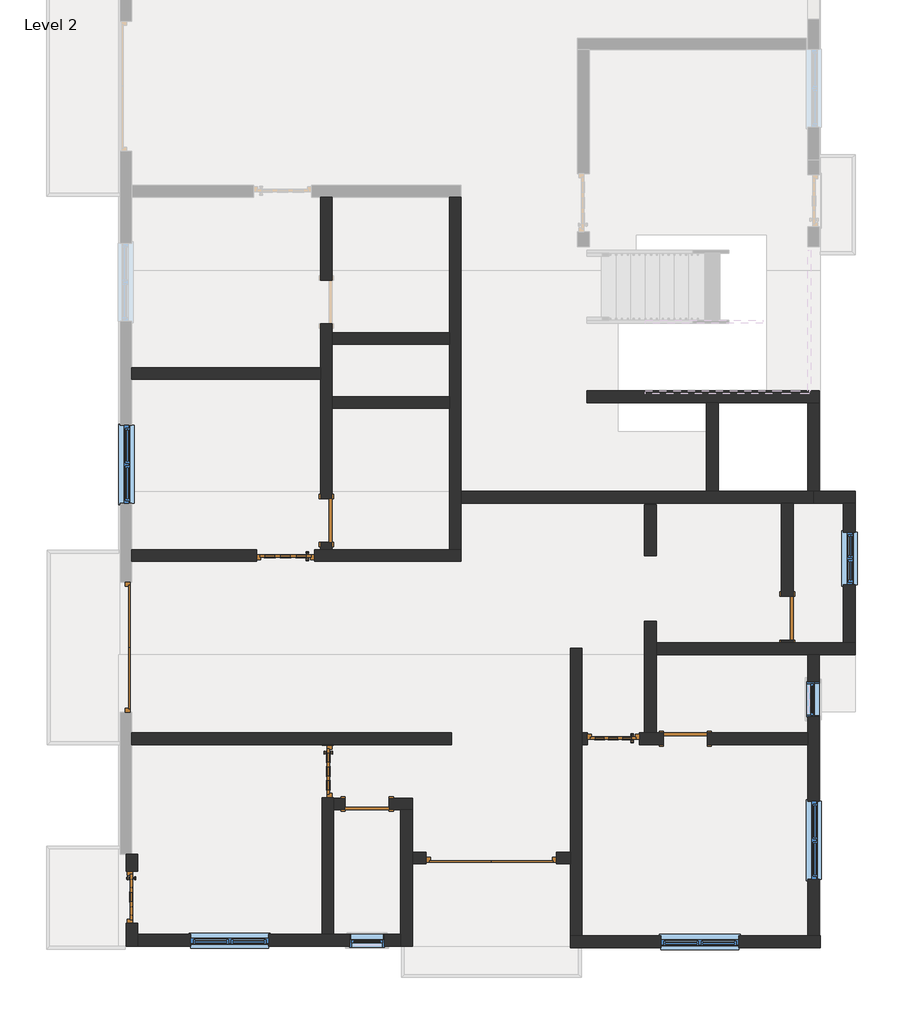
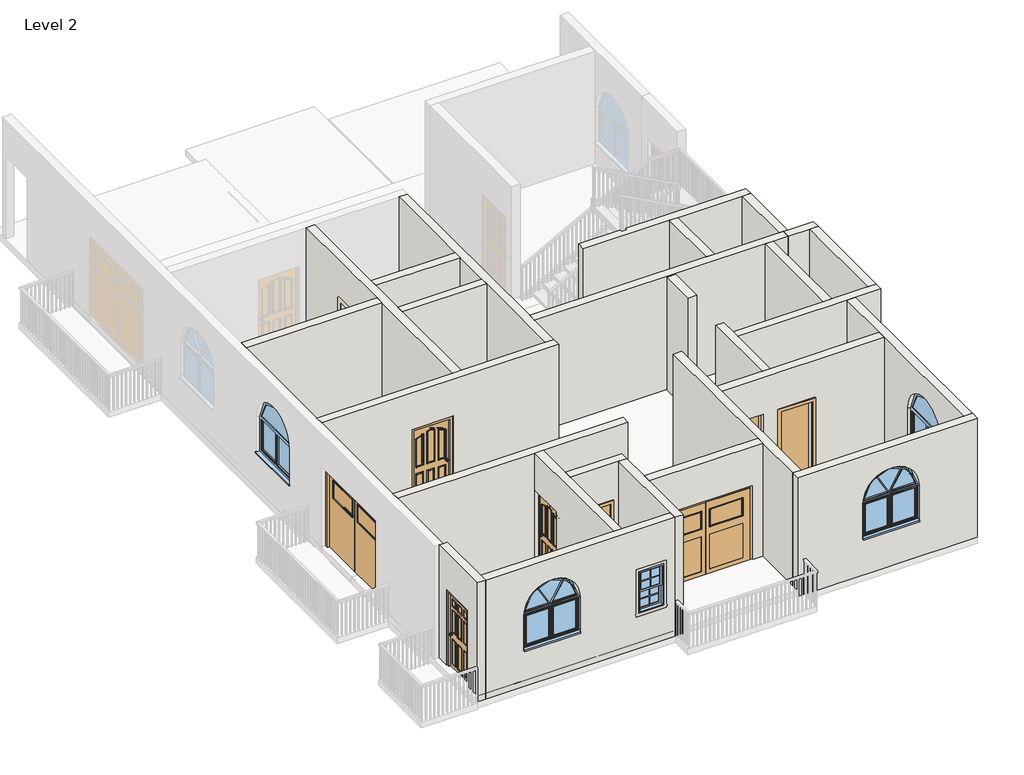
# One storey, part 1 of 7: 27 walls, 10 doors, 7 windows.
"""IFC4 building model written with IfcOpenShell, lengths in millimetres."""

from ifc_helpers import new_model, si_unit, frame, origin, place, context, project, spatial, polyline, circle_curve, outline, extrude, faceted_brep, transform, mapped, element, save
from ifc_brep_helpers import plane_surface, revolved_surface, advanced_brep
from components import doors_extsgl_5_910x2110mm_99758a98, doors_extsgl_6_1010x2110mm_b93c615f, doors_extsgl_6_1010x2110mm_efbaf1af, doors_extsgl_6_910x2110mm_72be2df1, doors_extsgl_6_910x2110mm_b26fcae4, doors_extsgl_6_910x2110mm_5dc58899, doors_extsgl_6_910x2110mm_16d7c084, doors_garage_timber_side_hung_glazing_2270x2050mm_ae99176d, doors_garage_timber_side_hung_glazing_2270x2200mm_badb7014, door_fadea3f2, door_53b1b562, window_679d2811, windows_arched_1360x910mm_c5754810, windows_dbl_w_glazing_bars_910x910mm_41eba874

model = new_model("IFC4")

# Units and contexts
model_context = context("Model", 3, world=origin())
ifc_project = project(units=[si_unit("LENGTHUNIT", "METRE", prefix="MILLI")], contexts=[model_context])

# Site, building, storey
site = spatial("IfcSite", under=ifc_project)
building = spatial("IfcBuilding", under=site)
storey = spatial("IfcBuildingStorey", under=building, Name="Level 2", Elevation=3048.0)

# Doors
placement = place(None, origin())
doors_extsgl_5_910x2110mm_shape = doors_extsgl_5_910x2110mm_99758a98(model_context)
element("IfcDoor", 1, ObjectType="Doors_ExtSgl_5 : 910x2110mm", at=placement, inside=storey, context=model_context, shape_type="MappedRepresentation", body=[
    mapped(doors_extsgl_5_910x2110mm_shape, transform((-6127.6013636, -9759.5108149, 3048.0), x_axis=(0.0, -1.0, 0.0), y_axis=(1.0, 0.0, 0.0), z_axis=(0.0, 0.0, 1.0))),
])
doors_extsgl_6_1010x2110mm_shape = doors_extsgl_6_1010x2110mm_b93c615f(model_context)
doors_extsgl_6_1010x2110mm_2_shape = doors_extsgl_6_1010x2110mm_efbaf1af(model_context)
element("IfcDoor", 2, ObjectType="Doors_ExtSgl_6 : 1010x2110mm", at=placement, inside=storey, context=model_context, shape_type="MappedRepresentation", body=[
    mapped(doors_extsgl_6_1010x2110mm_shape, transform((-3445.8775704, -3805.7037749, 3048.0), x_axis=(-1.0, 0.0, 0.0), y_axis=(0.0, -1.0, 0.0), z_axis=(0.0, 0.0, 1.0))),
    mapped(doors_extsgl_6_1010x2110mm_2_shape, transform((-3445.8775704, -3805.7037749, 3048.0), x_axis=(-1.0, 0.0, 0.0), y_axis=(0.0, -1.0, 0.0), z_axis=(0.0, 0.0, 1.0))),
])
doors_extsgl_6_910x2110mm_shape = doors_extsgl_6_910x2110mm_72be2df1(model_context)
doors_extsgl_6_910x2110mm_2_shape = doors_extsgl_6_910x2110mm_b26fcae4(model_context)
element("IfcDoor", 3, ObjectType="Doors_ExtSgl_6 : 910x2110mm", at=placement, inside=storey, context=model_context, shape_type="MappedRepresentation", body=[
    mapped(doors_extsgl_6_910x2110mm_shape, transform((2269.1224296, -6998.5466225, 3048.0), x_axis=(-1.0, 0.0, 0.0), y_axis=(0.0, -1.0, 0.0), z_axis=(0.0, 0.0, 1.0))),
    mapped(doors_extsgl_6_910x2110mm_2_shape, transform((2269.1224296, -6998.5466225, 3048.0), x_axis=(-1.0, 0.0, 0.0), y_axis=(0.0, -1.0, 0.0), z_axis=(0.0, 0.0, 1.0))),
])
doors_extsgl_6_910x2110mm_3_shape = doors_extsgl_6_910x2110mm_5dc58899(model_context)
doors_extsgl_6_910x2110mm_4_shape = doors_extsgl_6_910x2110mm_16d7c084(model_context)
element("IfcDoor", 4, ObjectType="Doors_ExtSgl_6 : 910x2110mm", at=placement, inside=storey, context=model_context, shape_type="MappedRepresentation", body=[
    mapped(doors_extsgl_6_910x2110mm_3_shape, transform((-2709.3109037, -7568.3747197, 3048.0), x_axis=(0.0, -1.0, 0.0), y_axis=(1.0, 0.0, 0.0), z_axis=(0.0, 0.0, 1.0))),
    mapped(doors_extsgl_6_910x2110mm_4_shape, transform((-2709.3109037, -7568.3747197, 3048.0), x_axis=(0.0, -1.0, 0.0), y_axis=(1.0, 0.0, 0.0), z_axis=(0.0, 0.0, 1.0))),
])
doors_garage_timber_side_hung_glazing_2270x2050mm_shape = doors_garage_timber_side_hung_glazing_2270x2050mm_ae99176d(model_context)
element("IfcDoor", 5, ObjectType="Doors_Garage_Timber_Side_Hung_Glazing : 2270x2050mm", at=placement, inside=storey, context=model_context, shape_type="MappedRepresentation", body=[
    mapped(doors_garage_timber_side_hung_glazing_2270x2050mm_shape, transform((141.8390963, -9078.0694836, 3048.0), x_axis=(-1.0, 0.0, 0.0), y_axis=(0.0, -1.0, 0.0), z_axis=(0.0, 0.0, 1.0))),
])
doors_garage_timber_side_hung_glazing_2270x2200mm_shape = doors_garage_timber_side_hung_glazing_2270x2200mm_badb7014(model_context)
element("IfcDoor", 6, ObjectType="Doors_Garage_Timber_Side_Hung_Glazing : 2270x2200mm", at=placement, inside=storey, context=model_context, shape_type="MappedRepresentation", body=[
    mapped(doors_garage_timber_side_hung_glazing_2270x2200mm_shape, transform((-6229.2013636, -5402.1251987, 3048.0), x_axis=(0.0, 1.0, 0.0), y_axis=(-1.0, 0.0, 0.0), z_axis=(0.0, 0.0, 1.0))),
])
door_shape = door_fadea3f2(model_context)
element("IfcDoor", 7, ObjectType="Single-Flush : 30\" x 80\"", at=placement, inside=storey, context=model_context, shape_type="MappedRepresentation", body=[
    mapped(door_shape, transform((-2023.5109037, -8138.2694836, 3048.0), x_axis=(-1.0, 0.0, 0.0), y_axis=(0.0, -1.0, 0.0), z_axis=(0.0, 0.0, 1.0))),
])
element("IfcDoor", 8, ObjectType="Single-Flush : 30\" x 80\"", at=placement, inside=storey, context=model_context, shape_type="MappedRepresentation", body=[
    mapped(door_shape, transform((5304.3890963, -4897.9037749, 3048.0), x_axis=(0.0, -1.0, 0.0), y_axis=(1.0, 0.0, 0.0), z_axis=(0.0, 0.0, 1.0))),
])
door_2_shape = door_53b1b562(model_context)
element("IfcDoor", 9, ObjectType="Single-Flush : 30\" x 80\"", at=placement, inside=storey, context=model_context, shape_type="MappedRepresentation", body=[
    mapped(door_2_shape, transform((-2734.7109037, -3196.1037749, 3048.0), x_axis=(0.0, 1.0, 0.0), y_axis=(-1.0, 0.0, 0.0), z_axis=(0.0, 0.0, 1.0))),
])
element("IfcDoor", 10, ObjectType="Single-Flush : 30\" x 80\"", at=placement, inside=storey, context=model_context, shape_type="MappedRepresentation", body=[
    mapped(door_2_shape, transform((3526.3890963, -6998.5466225, 3048.0), x_axis=(-1.0, 0.0, 0.0), y_axis=(0.0, -1.0, 0.0), z_axis=(0.0, 0.0, 1.0))),
])

# Walls
element("IfcWall", 11, ObjectType="Generic - 9\" w", at=placement, inside=storey, context=model_context, shape_type="Brep", body=[
    faceted_brep([(6485.4890963, -2688.1037749, 3048.0), (5863.1890963, -2688.1037749, 3048.0), (5761.5890963, -2688.1037749, 3048.0), (5761.5890963, -2688.1037749, 6096.0), (5863.1890963, -2688.1037749, 6096.0), (6485.4890963, -2688.1037749, 6096.0), (6485.4890963, -2891.3037749, 3048.0), (6485.4890963, -2891.3037749, 6096.0), (6282.2890963, -2891.3037749, 6096.0), (5761.5890963, -2891.3037749, 6096.0), (5761.5890963, -2891.3037749, 3048.0), (6282.2890963, -2891.3037749, 3048.0)], [[[0, 1, 2, 3, 4, 5]], [[6, 7, 8, 9, 10, 11]], [[2, 1, 0, 6, 11, 10]], [[3, 2, 10, 9]], [[5, 4, 3, 9, 8, 7]], [[0, 5, 7, 6]]]),
])
element("IfcWall", 12, ObjectType="Generic - 9\" w", at=placement, inside=storey, context=model_context, shape_type="Brep", body=[
    faceted_brep([(5761.5890963, -2688.1037749, 3048.0), (5659.9890963, -2688.1037749, 3048.0), (4097.8890963, -2688.1037749, 3048.0), (3894.6890963, -2688.1037749, 3048.0), (-385.2109037, -2688.1037749, 3048.0), (-385.2109037, -2688.1037749, 6096.0), (3894.6890963, -2688.1037749, 6096.0), (4097.8890963, -2688.1037749, 6096.0), (5659.9890963, -2688.1037749, 6096.0), (5761.5890963, -2688.1037749, 6096.0), (5761.5890963, -2891.3037749, 3048.0), (5761.5890963, -2891.3037749, 6096.0), (5405.9890963, -2891.3037749, 6096.0), (5202.7890963, -2891.3037749, 6096.0), (-385.2109037, -2891.3037749, 6096.0), (-385.2109037, -2891.3037749, 3048.0), (5202.7890963, -2891.3037749, 3048.0), (5405.9890963, -2891.3037749, 3048.0)], [[[0, 1, 2, 3, 4, 5, 6, 7, 8, 9]], [[10, 11, 12, 13, 14, 15, 16, 17]], [[4, 3, 2, 1, 0, 10, 17, 16, 15]], [[9, 8, 7, 6, 5, 14, 13, 12, 11]], [[0, 9, 11, 10]], [[5, 4, 15, 14]]]),
])
element("IfcWall", 13, ObjectType="Generic - 9\" w", at=placement, inside=storey, context=model_context, shape_type="SweptSolid", body=[
    extrude(outline(polyline([(3894.6890963, -2688.1037749), (3894.6890963, -1138.7037749), (4097.8890963, -1138.7037749), (4097.8890963, -2688.1037749), (3894.6890963, -2688.1037749)])), frame((0.0, 0.0, 3048.0), z_axis=(0.0, 0.0, 1.0), x_axis=(1.0, 0.0, 0.0)), (0.0, 0.0, 1.0), 3048.0),
])
element("IfcWall", 14, ObjectType="Generic - 9\" w", at=placement, inside=storey, context=model_context, shape_type="Brep", body=[
    faceted_brep([(5863.1890963, -935.5037749, 3048.0), (1812.4805171, -935.5037749, 3048.0), (1812.4805171, -935.5037749, 6096.0), (5863.1890963, -935.5037749, 6096.0), (5863.1890963, -1138.7037749, 3048.0), (5863.1890963, -1138.7037749, 6096.0), (5659.9890963, -1138.7037749, 6096.0), (4097.8890963, -1138.7037749, 6096.0), (3894.6890963, -1138.7037749, 6096.0), (1812.4805171, -1138.7037749, 6096.0), (1812.4805171, -1138.7037749, 3048.0), (3894.6890963, -1138.7037749, 3048.0), (4097.8890963, -1138.7037749, 3048.0), (5659.9890963, -1138.7037749, 3048.0)], [[[0, 1, 2, 3]], [[4, 5, 6, 7, 8, 9, 10, 11, 12, 13]], [[1, 0, 4, 13, 12, 11, 10]], [[2, 1, 10, 9]], [[3, 2, 9, 8, 7, 6, 5]], [[0, 3, 5, 4]]]),
])
element("IfcWall", 15, ObjectType="Generic - 9\" w", at=placement, inside=storey, context=model_context, shape_type="AdvancedBrep", body=[
    advanced_brep(
    [(1519.7890963, -10638.3037749, 3048.0), (5875.8890963, -10638.3037749, 3048.0), (5875.8890963, -10638.3037749, 6096.0), (1519.7890963, -10638.3037749, 6096.0), (4460.3890963, -10638.3037749, 3962.4), (3100.3890963, -10638.3037749, 3962.4), (3100.3890963, -10638.3037749, 4872.4), (4460.3890963, -10638.3037749, 4872.4), (1519.7890963, -10435.1037749, 3048.0), (1519.7890963, -10435.1037749, 6096.0), (1722.9890963, -10435.1037749, 6096.0), (5659.9890963, -10435.1037749, 6096.0), (5863.1890963, -10435.1037749, 6096.0), (5875.8890963, -10435.1037749, 6096.0), (5875.8890963, -10435.1037749, 3048.0), (5863.1890963, -10435.1037749, 3048.0), (5659.9890963, -10435.1037749, 3048.0), (1722.9890963, -10435.1037749, 3048.0), (4460.3890963, -10435.1037749, 3962.4), (4460.3890963, -10435.1037749, 4872.4), (3100.3890963, -10435.1037749, 4872.4), (3100.3890963, -10435.1037749, 3962.4)],
    [
        (0, 1),
        (1, 2),
        (2, 3),
        (3, 0),
        (4, 5),
        (5, 6),
        (6, 7, circle_curve(frame((3780.3890963, -10638.3037749, 4872.4), z_axis=(0.0, 1.0, 0.0), x_axis=(-1.0, 0.0, 0.0)), 680.0)),
        (7, 4),
        (8, 9),
        (9, 10),
        (10, 11),
        (11, 12),
        (12, 13),
        (13, 14),
        (14, 15),
        (15, 16),
        (16, 17),
        (17, 8),
        (18, 19),
        (19, 20, circle_curve(frame((3780.3890963, -10435.1037749, 4872.4), z_axis=(0.0, -1.0, 0.0), x_axis=(-1.0, 0.0, 0.0)), 680.0)),
        (20, 21),
        (21, 18),
        (0, 8),
        (14, 1),
        (13, 2),
        (9, 3),
        (18, 4),
        (7, 19),
        (6, 20),
        (5, 21),
    ],
    [
        plane_surface(frame((1722.9890963, -10638.3037749, 3048.0), z_axis=(0.0, -1.0, 0.0), x_axis=(1.0, 0.0, 0.0))),
        plane_surface(frame((1722.9890963, -10435.1037749, 3048.0), z_axis=(0.0, 1.0, 0.0), x_axis=(-1.0, 0.0, 0.0))),
        plane_surface(frame((1621.3890963, -10638.3037749, 3048.0), z_axis=(0.0, 0.0, -1.0), x_axis=(0.0, 1.0, 0.0))),
        plane_surface(frame((5875.8890963, -10638.3037749, 3048.0), z_axis=(1.0, 0.0, 0.0), x_axis=(0.0, 1.0, 0.0))),
        plane_surface(frame((5875.8890963, -10638.3037749, 6096.0), z_axis=(0.0, 0.0, 1.0), x_axis=(0.0, 1.0, 0.0))),
        plane_surface(frame((1519.7890963, -5418.6037749, 3048.0), z_axis=(-1.0, 0.0, 0.0), x_axis=(0.0, -1.0, 0.0))),
        plane_surface(frame((4460.3890963, -10435.1037749, 3962.4), z_axis=(-1.0, 0.0, 0.0), x_axis=(0.0, -1.0, 0.0))),
        revolved_surface(polyline([(3100.3890963, -10638.3037749, 4872.4), (3100.3890963, -10435.1037749, 4872.4)]), (3780.3890963, -10435.1037749, 4872.4), (0.0, -1.0, 0.0)),
        plane_surface(frame((3100.3890963, -10435.1037749, 4872.4), z_axis=(1.0, 0.0, 0.0), x_axis=(0.0, -1.0, 0.0))),
        plane_surface(frame((3100.3890963, -10435.1037749, 3962.4), z_axis=(0.0, 0.0, 1.0), x_axis=(0.0, -1.0, 0.0))),
    ],
    [
        (0, [[1, 2, 3, 4], [5, 6, 7, 8]]),
        (1, [[9, 10, 11, 12, 13, 14, 15, 16, 17, 18], [19, 20, 21, 22]]),
        (2, [[-1, 23, -18, -17, -16, -15, 24]]),
        (3, [[-2, -24, -14, 25]]),
        (4, [[-3, -25, -13, -12, -11, -10, 26]]),
        (5, [[-4, -26, -9, -23]]),
        (6, [[-19, 27, -8, 28]]),
        (7, [[-20, -28, -7, 29]]),
        (8, [[-21, -29, -6, 30]]),
        (9, [[-22, -30, -5, -27]]),
    ],
),
])
element("IfcWall", 16, ObjectType="Generic - 9\" w", at=placement, inside=storey, context=model_context, shape_type="AdvancedBrep", body=[
    advanced_brep(
    [(5863.1890963, -10435.1037749, 3048.0), (5863.1890963, -5532.9037749, 3048.0), (5863.1890963, -5532.9037749, 6096.0), (5863.1890963, -10435.1037749, 6096.0), (5863.1890963, -8087.6251987, 3962.4), (5863.1890963, -9447.6251987, 3962.4), (5863.1890963, -9447.6251987, 4872.4), (5863.1890963, -8087.6251987, 4872.4), (5863.1890963, -6618.7537749, 5029.2), (5863.1890963, -6009.1537749, 5029.2), (5863.1890963, -6009.1537749, 3962.4), (5863.1890963, -6618.7537749, 3962.4), (5659.9890963, -10435.1037749, 3048.0), (5659.9890963, -10435.1037749, 6096.0), (5659.9890963, -7100.1466225, 6096.0), (5659.9890963, -6896.9466225, 6096.0), (5659.9890963, -5532.9037749, 6096.0), (5659.9890963, -5532.9037749, 3048.0), (5659.9890963, -6896.9466225, 3048.0), (5659.9890963, -7100.1466225, 3048.0), (5659.9890963, -8087.6251987, 3962.4), (5659.9890963, -8087.6251987, 4872.4), (5659.9890963, -9447.6251987, 4872.4), (5659.9890963, -9447.6251987, 3962.4), (5659.9890963, -6618.7537749, 5029.2), (5659.9890963, -6618.7537749, 3962.4), (5659.9890963, -6009.1537749, 3962.4), (5659.9890963, -6009.1537749, 5029.2)],
    [
        (0, 1),
        (1, 2),
        (2, 3),
        (3, 0),
        (4, 5),
        (5, 6),
        (6, 7, circle_curve(frame((5863.1890963, -8767.6251987, 4872.4), z_axis=(-1.0, 0.0, 0.0), x_axis=(0.0, -1.0, 0.0)), 680.0)),
        (7, 4),
        (8, 9),
        (9, 10),
        (10, 11),
        (11, 8),
        (12, 13),
        (13, 14),
        (14, 15),
        (15, 16),
        (16, 17),
        (17, 18),
        (18, 19),
        (19, 12),
        (20, 21),
        (21, 22, circle_curve(frame((5659.9890963, -8767.6251987, 4872.4), z_axis=(1.0, 0.0, 0.0), x_axis=(0.0, -1.0, 0.0)), 680.0)),
        (22, 23),
        (23, 20),
        (24, 25),
        (25, 26),
        (26, 27),
        (27, 24),
        (0, 12),
        (17, 1),
        (2, 16),
        (13, 3),
        (20, 4),
        (7, 21),
        (6, 22),
        (5, 23),
        (24, 8),
        (11, 25),
        (10, 26),
        (9, 27),
    ],
    [
        plane_surface(frame((5863.1890963, -10435.1037749, 3048.0), z_axis=(1.0, 0.0, 0.0), x_axis=(0.0, 1.0, 0.0))),
        plane_surface(frame((5659.9890963, -10435.1037749, 3048.0), z_axis=(-1.0, 0.0, 0.0), x_axis=(0.0, -1.0, 0.0))),
        plane_surface(frame((5863.1890963, -10536.7037749, 3048.0), z_axis=(0.0, 0.0, -1.0), x_axis=(-1.0, 0.0, 0.0))),
        plane_surface(frame((5863.1890963, -5431.3037749, 6096.0), z_axis=(0.0, 0.0, 1.0), x_axis=(-1.0, 0.0, 0.0))),
        plane_surface(frame((1722.9890963, -10435.1037749, 3048.0), z_axis=(0.0, -1.0, 0.0), x_axis=(-1.0, 0.0, 0.0))),
        plane_surface(frame((3018.3890963, -5532.9037749, 3048.0), z_axis=(0.0, 1.0, 0.0), x_axis=(1.0, 0.0, 0.0))),
        plane_surface(frame((5659.9890963, -8087.6251987, 3962.4), z_axis=(0.0, -1.0, 0.0), x_axis=(1.0, 0.0, 0.0))),
        revolved_surface(polyline([(5863.1890963, -9447.6251987, 4872.4), (5659.9890963, -9447.6251987, 4872.4)]), (5659.9890963, -8767.6251987, 4872.4), (1.0, 0.0, 0.0)),
        plane_surface(frame((5659.9890963, -9447.6251987, 4872.4), z_axis=(0.0, 1.0, 0.0), x_axis=(1.0, 0.0, 0.0))),
        plane_surface(frame((5659.9890963, -9447.6251987, 3962.4), z_axis=(0.0, 0.0, 1.0), x_axis=(1.0, 0.0, 0.0))),
        plane_surface(frame((5659.9890963, -6618.7537749, 5029.2), z_axis=(0.0, 1.0, 0.0), x_axis=(1.0, 0.0, 0.0))),
        plane_surface(frame((5659.9890963, -6618.7537749, 3962.4), z_axis=(0.0, 0.0, 1.0), x_axis=(1.0, 0.0, 0.0))),
        plane_surface(frame((5659.9890963, -6009.1537749, 3962.4), z_axis=(0.0, -1.0, 0.0), x_axis=(1.0, 0.0, 0.0))),
        plane_surface(frame((5659.9890963, -6009.1537749, 5029.2), z_axis=(0.0, 0.0, -1.0), x_axis=(1.0, 0.0, 0.0))),
    ],
    [
        (0, [[1, 2, 3, 4], [5, 6, 7, 8], [9, 10, 11, 12]]),
        (1, [[13, 14, 15, 16, 17, 18, 19, 20], [21, 22, 23, 24], [25, 26, 27, 28]]),
        (2, [[-1, 29, -20, -19, -18, 30]]),
        (3, [[-3, 31, -16, -15, -14, 32]]),
        (4, [[-4, -32, -13, -29]]),
        (5, [[-2, -30, -17, -31]]),
        (6, [[-21, 33, -8, 34]]),
        (7, [[-22, -34, -7, 35]]),
        (8, [[-23, -35, -6, 36]]),
        (9, [[-24, -36, -5, -33]]),
        (10, [[-25, 37, -12, 38]]),
        (11, [[-26, -38, -11, 39]]),
        (12, [[-27, -39, -10, 40]]),
        (13, [[-28, -40, -9, -37]]),
    ],
),
])
element("IfcWall", 17, ObjectType="Generic - 9\" w", at=placement, inside=storey, context=model_context, shape_type="Brep", body=[
    faceted_brep([(5659.9890963, -1138.7037749, 3048.0), (5659.9890963, -2688.1037749, 3048.0), (5659.9890963, -2688.1037749, 6096.0), (5659.9890963, -1138.7037749, 6096.0), (5863.1890963, -1138.7037749, 3048.0), (5863.1890963, -1138.7037749, 6096.0), (5863.1890963, -2688.1037749, 6096.0), (5863.1890963, -2688.1037749, 3048.0), (5761.5890963, -2688.1037749, 3048.0), (5761.5890963, -2688.1037749, 6096.0)], [[[0, 1, 2, 3]], [[4, 5, 6, 7]], [[1, 0, 4, 7, 8]], [[3, 2, 9, 6, 5]], [[2, 1, 8, 7, 6, 9]], [[0, 3, 5, 4]]]),
])
element("IfcWall", 18, ObjectType="Generic - 9\" w", at=placement, inside=storey, context=model_context, shape_type="Brep", body=[
    faceted_brep([(-6229.2013636, -10214.5441482, 5158.0), (-6229.2013636, -10214.5441482, 3048.0), (-6229.2013636, -10612.9037749, 3048.0), (-6229.2013636, -10612.9037749, 6096.0), (-6229.2013636, -9007.7845215, 6096.0), (-6229.2013636, -9007.7845215, 3048.0), (-6229.2013636, -9304.5441482, 3048.0), (-6229.2013636, -9304.5441482, 5158.0), (-6026.0013636, -10612.9037749, 3048.0), (-6026.0013636, -10409.7037749, 3048.0), (-6026.0013636, -10214.5441482, 3048.0), (-6026.0013636, -10214.5441482, 5158.0), (-6026.0013636, -9304.5441482, 5158.0), (-6026.0013636, -9304.5441482, 3048.0), (-6026.0013636, -9007.7845215, 3048.0), (-6026.0013636, -9007.7845215, 6096.0), (-6026.0013636, -10409.7037749, 6096.0), (-6026.0013636, -10612.9037749, 6096.0), (-6127.6013636, -9007.7845215, 3048.0), (-6127.6013636, -9007.7845215, 6096.0)], [[[0, 1, 2, 3, 4, 5, 6, 7]], [[8, 9, 10, 11, 12, 13, 14, 15, 16, 17]], [[6, 5, 18, 14, 13]], [[2, 1, 10, 9, 8]], [[4, 3, 17, 16, 15, 19]], [[5, 4, 19, 15, 14, 18]], [[13, 12, 7, 6]], [[11, 10, 1, 0]], [[12, 11, 0, 7]], [[3, 2, 8, 17]]]),
])
element("IfcWall", 19, ObjectType="Generic - 9\" w", at=placement, inside=storey, context=model_context, shape_type="AdvancedBrep", body=[
    advanced_brep(
    [(-6026.0013636, -10612.9037749, 3048.0), (-1439.3109037, -10612.9037749, 3048.0), (-1439.3109037, -10612.9037749, 6096.0), (-6026.0013636, -10612.9037749, 6096.0), (-3738.4561337, -10612.9037749, 3962.4), (-5098.4561337, -10612.9037749, 3962.4), (-5098.4561337, -10612.9037749, 4872.4), (-3738.4561337, -10612.9037749, 4872.4), (-1718.7109037, -10612.9037749, 5029.2), (-1718.7109037, -10612.9037749, 3962.4), (-2328.3109037, -10612.9037749, 3962.4), (-2328.3109037, -10612.9037749, 5029.2), (-6026.0013636, -10409.7037749, 3048.0), (-6026.0013636, -10409.7037749, 6096.0), (-2810.9109037, -10409.7037749, 6096.0), (-2607.7109037, -10409.7037749, 6096.0), (-1439.3109037, -10409.7037749, 6096.0), (-1439.3109037, -10409.7037749, 3048.0), (-2607.7109037, -10409.7037749, 3048.0), (-2810.9109037, -10409.7037749, 3048.0), (-3738.4561337, -10409.7037749, 3962.4), (-3738.4561337, -10409.7037749, 4872.4), (-5098.4561337, -10409.7037749, 4872.4), (-5098.4561337, -10409.7037749, 3962.4), (-1718.7109037, -10409.7037749, 5029.2), (-2328.3109037, -10409.7037749, 5029.2), (-2328.3109037, -10409.7037749, 3962.4), (-1718.7109037, -10409.7037749, 3962.4)],
    [
        (0, 1),
        (1, 2),
        (2, 3),
        (3, 0),
        (4, 5),
        (5, 6),
        (6, 7, circle_curve(frame((-4418.4561337, -10612.9037749, 4872.4), z_axis=(0.0, 1.0, 0.0), x_axis=(-1.0, 0.0, 0.0)), 680.0)),
        (7, 4),
        (8, 9),
        (9, 10),
        (10, 11),
        (11, 8),
        (12, 13),
        (13, 14),
        (14, 15),
        (15, 16),
        (16, 17),
        (17, 18),
        (18, 19),
        (19, 12),
        (20, 21),
        (21, 22, circle_curve(frame((-4418.4561337, -10409.7037749, 4872.4), z_axis=(0.0, -1.0, 0.0), x_axis=(-1.0, 0.0, 0.0)), 680.0)),
        (22, 23),
        (23, 20),
        (24, 25),
        (25, 26),
        (26, 27),
        (27, 24),
        (0, 12),
        (17, 1),
        (2, 16),
        (13, 3),
        (20, 4),
        (7, 21),
        (6, 22),
        (5, 23),
        (8, 24),
        (27, 9),
        (26, 10),
        (25, 11),
    ],
    [
        plane_surface(frame((-6229.2013636, -10612.9037749, 3048.0), z_axis=(0.0, -1.0, 0.0), x_axis=(1.0, 0.0, 0.0))),
        plane_surface(frame((-6229.2013636, -10409.7037749, 3048.0), z_axis=(0.0, 1.0, 0.0), x_axis=(-1.0, 0.0, 0.0))),
        plane_surface(frame((-6127.6013636, -10612.9037749, 3048.0), z_axis=(0.0, 0.0, -1.0), x_axis=(0.0, 1.0, 0.0))),
        plane_surface(frame((-1337.7109037, -10612.9037749, 6096.0), z_axis=(0.0, 0.0, 1.0), x_axis=(0.0, 1.0, 0.0))),
        plane_surface(frame((-1439.3109037, -8239.8694836, 3048.0), z_axis=(1.0, 0.0, 0.0), x_axis=(0.0, -1.0, 0.0))),
        plane_surface(frame((-6026.0013636, -9109.3845215, 3048.0), z_axis=(-1.0, 0.0, 0.0), x_axis=(0.0, 1.0, 0.0))),
        plane_surface(frame((-3738.4561337, -10409.7037749, 3962.4), z_axis=(-1.0, 0.0, 0.0), x_axis=(0.0, -1.0, 0.0))),
        revolved_surface(polyline([(-5098.4561337, -10612.9037749, 4872.4), (-5098.4561337, -10409.7037749, 4872.4)]), (-4418.4561337, -10409.7037749, 4872.4), (0.0, -1.0, 0.0)),
        plane_surface(frame((-5098.4561337, -10409.7037749, 4872.4), z_axis=(1.0, 0.0, 0.0), x_axis=(0.0, -1.0, 0.0))),
        plane_surface(frame((-5098.4561337, -10409.7037749, 3962.4), z_axis=(0.0, 0.0, 1.0), x_axis=(0.0, -1.0, 0.0))),
        plane_surface(frame((-1718.7109037, -10612.9037749, 5029.2), z_axis=(-1.0, 0.0, 0.0), x_axis=(0.0, 1.0, 0.0))),
        plane_surface(frame((-1718.7109037, -10612.9037749, 3962.4), z_axis=(0.0, 0.0, 1.0), x_axis=(0.0, 1.0, 0.0))),
        plane_surface(frame((-2328.3109037, -10612.9037749, 3962.4), z_axis=(1.0, 0.0, 0.0), x_axis=(0.0, 1.0, 0.0))),
        plane_surface(frame((-2328.3109037, -10612.9037749, 5029.2), z_axis=(0.0, 0.0, -1.0), x_axis=(0.0, 1.0, 0.0))),
    ],
    [
        (0, [[1, 2, 3, 4], [5, 6, 7, 8], [9, 10, 11, 12]]),
        (1, [[13, 14, 15, 16, 17, 18, 19, 20], [21, 22, 23, 24], [25, 26, 27, 28]]),
        (2, [[-1, 29, -20, -19, -18, 30]]),
        (3, [[-3, 31, -16, -15, -14, 32]]),
        (4, [[-2, -30, -17, -31]]),
        (5, [[-4, -32, -13, -29]]),
        (6, [[-21, 33, -8, 34]]),
        (7, [[-22, -34, -7, 35]]),
        (8, [[-23, -35, -6, 36]]),
        (9, [[-24, -36, -5, -33]]),
        (10, [[-9, 37, -28, 38]]),
        (11, [[-10, -38, -27, 39]]),
        (12, [[-11, -39, -26, 40]]),
        (13, [[-12, -40, -25, -37]]),
    ],
),
])
element("IfcWall", 20, ObjectType="Generic -4.5\" p", at=placement, inside=storey, context=model_context, shape_type="Brep", body=[
    faceted_brep([(-2836.3109037, 232.8962251, 3048.0), (-2836.3109037, -529.1037749, 3048.0), (-2836.3109037, -732.3037749, 3048.0), (-2836.3109037, -2815.1037749, 3048.0), (-2836.3109037, -2815.1037749, 5080.0), (-2836.3109037, -3577.1037749, 5080.0), (-2836.3109037, -3577.1037749, 3048.0), (-2836.3109037, -3704.1037749, 3048.0), (-2836.3109037, -3704.1037749, 6096.0), (-2836.3109037, -732.3037749, 6096.0), (-2836.3109037, -529.1037749, 6096.0), (-2836.3109037, 2442.6962251, 6096.0), (-2836.3109037, 2442.6962251, 3048.0), (-2836.3109037, 994.8962251, 3048.0), (-2836.3109037, 994.8962251, 5080.0), (-2836.3109037, 232.8962251, 5080.0), (-2633.1109037, -2815.1037749, 5080.0), (-2633.1109037, -2815.1037749, 3048.0), (-2633.1109037, -1240.3037749, 3048.0), (-2633.1109037, -1037.1037749, 3048.0), (-2633.1109037, -122.7037749, 3048.0), (-2633.1109037, 80.4962251, 3048.0), (-2633.1109037, 232.8962251, 3048.0), (-2633.1109037, 232.8962251, 5080.0), (-2633.1109037, 994.8962251, 5080.0), (-2633.1109037, 994.8962251, 3048.0), (-2633.1109037, 2442.6962251, 3048.0), (-2633.1109037, 2442.6962251, 6096.0), (-2633.1109037, 80.4962251, 6096.0), (-2633.1109037, -122.7037749, 6096.0), (-2633.1109037, -1037.1037749, 6096.0), (-2633.1109037, -1240.3037749, 6096.0), (-2633.1109037, -3704.1037749, 6096.0), (-2633.1109037, -3704.1037749, 3048.0), (-2633.1109037, -3577.1037749, 3048.0), (-2633.1109037, -3577.1037749, 5080.0)], [[[0, 1, 2, 3, 4, 5, 6, 7, 8, 9, 10, 11, 12, 13, 14, 15]], [[16, 17, 18, 19, 20, 21, 22, 23, 24, 25, 26, 27, 28, 29, 30, 31, 32, 33, 34, 35]], [[26, 25, 13, 12]], [[34, 33, 7, 6]], [[22, 21, 20, 19, 18, 17, 3, 2, 1, 0]], [[11, 10, 9, 8, 32, 31, 30, 29, 28, 27]], [[12, 11, 27, 26]], [[8, 7, 33, 32]], [[14, 13, 25, 24]], [[15, 14, 24, 23]], [[0, 15, 23, 22]], [[4, 3, 17, 16]], [[5, 4, 16, 35]], [[6, 5, 35, 34]]]),
])
element("IfcWall", 21, ObjectType="Generic -4.5\" p", at=placement, inside=storey, context=model_context, shape_type="Brep", body=[
    faceted_brep([(-6127.6013636, -3907.3037749, 3048.0), (-3950.9109037, -3907.3037749, 3048.0), (-3950.9109037, -3907.3037749, 5158.0), (-2940.9109037, -3907.3037749, 5158.0), (-2940.9109037, -3907.3037749, 3048.0), (-385.2109037, -3907.3037749, 3048.0), (-385.2109037, -3907.3037749, 6096.0), (-6127.6013636, -3907.3037749, 6096.0), (-3950.9109037, -3704.1037749, 5158.0), (-3950.9109037, -3704.1037749, 3048.0), (-6127.6013636, -3704.1037749, 3048.0), (-6127.6013636, -3704.1037749, 6096.0), (-2836.3109037, -3704.1037749, 6096.0), (-2633.1109037, -3704.1037749, 6096.0), (-588.4109037, -3704.1037749, 6096.0), (-385.2109037, -3704.1037749, 6096.0), (-385.2109037, -3704.1037749, 3048.0), (-588.4109037, -3704.1037749, 3048.0), (-2633.1109037, -3704.1037749, 3048.0), (-2836.3109037, -3704.1037749, 3048.0), (-2940.9109037, -3704.1037749, 3048.0), (-2940.9109037, -3704.1037749, 5158.0)], [[[0, 1, 2, 3, 4, 5, 6, 7]], [[8, 9, 10, 11, 12, 13, 14, 15, 16, 17, 18, 19, 20, 21]], [[10, 9, 1, 0]], [[20, 19, 18, 17, 16, 5, 4]], [[7, 6, 15, 14, 13, 12, 11]], [[6, 5, 16, 15]], [[4, 3, 21, 20]], [[2, 1, 9, 8]], [[3, 2, 8, 21]], [[0, 7, 11, 10]]]),
])
element("IfcWall", 22, ObjectType="Generic -4.5\" p", at=placement, inside=storey, context=model_context, shape_type="Brep", body=[
    faceted_brep([(-385.2109037, -3704.1037749, 3048.0), (-385.2109037, -2891.3037749, 3048.0), (-385.2109037, -2688.1037749, 3048.0), (-385.2109037, 2442.6962251, 3048.0), (-385.2109037, 2442.6962251, 6096.0), (-385.2109037, -2688.1037749, 6096.0), (-385.2109037, -2891.3037749, 6096.0), (-385.2109037, -3704.1037749, 6096.0), (-588.4109037, -3704.1037749, 3048.0), (-588.4109037, -3704.1037749, 6096.0), (-588.4109037, -1240.3037749, 6096.0), (-588.4109037, -1037.1037749, 6096.0), (-588.4109037, -122.7037749, 6096.0), (-588.4109037, 80.4962251, 6096.0), (-588.4109037, 2442.6962251, 6096.0), (-588.4109037, 2442.6962251, 3048.0), (-588.4109037, 80.4962251, 3048.0), (-588.4109037, -122.7037749, 3048.0), (-588.4109037, -1037.1037749, 3048.0), (-588.4109037, -1240.3037749, 3048.0)], [[[0, 1, 2, 3, 4, 5, 6, 7]], [[8, 9, 10, 11, 12, 13, 14, 15, 16, 17, 18, 19]], [[3, 2, 1, 0, 8, 19, 18, 17, 16, 15]], [[7, 6, 5, 4, 14, 13, 12, 11, 10, 9]], [[4, 3, 15, 14]], [[0, 7, 9, 8]]]),
])
element("IfcWall", 23, ObjectType="Generic -4.5\" p", at=placement, inside=storey, context=model_context, shape_type="SweptSolid", body=[
    extrude(outline(polyline([(-588.4109037, -122.7037749), (-2633.1109037, -122.7037749), (-2633.1109037, 80.4962251), (-588.4109037, 80.4962251), (-588.4109037, -122.7037749)])), frame((0.0, 0.0, 3048.0), z_axis=(0.0, 0.0, 1.0), x_axis=(1.0, 0.0, 0.0)), (0.0, 0.0, 1.0), 3048.0),
])
element("IfcWall", 24, ObjectType="Generic -4.5\" p", at=placement, inside=storey, context=model_context, shape_type="SweptSolid", body=[
    extrude(outline(polyline([(-2836.3109037, -732.3037749), (-6127.6013636, -732.3037749), (-6127.6013636, -529.1037749), (-2836.3109037, -529.1037749), (-2836.3109037, -732.3037749)])), frame((0.0, 0.0, 3048.0), z_axis=(0.0, 0.0, 1.0), x_axis=(1.0, 0.0, 0.0)), (0.0, 0.0, 1.0), 3048.0),
])
element("IfcWall", 25, ObjectType="Generic -4.5\" p", at=placement, inside=storey, context=model_context, shape_type="SweptSolid", body=[
    extrude(outline(polyline([(-588.4109037, -1240.3037749), (-2633.1109037, -1240.3037749), (-2633.1109037, -1037.1037749), (-588.4109037, -1037.1037749), (-588.4109037, -1240.3037749)])), frame((0.0, 0.0, 3048.0), z_axis=(0.0, 0.0, 1.0), x_axis=(1.0, 0.0, 0.0)), (0.0, 0.0, 1.0), 3048.0),
])
element("IfcWall", 26, ObjectType="Generic -4.5\" p", at=placement, inside=storey, context=model_context, shape_type="Brep", body=[
    faceted_brep([(-6127.6013636, -7100.1466225, 3048.0), (-2810.9109037, -7100.1466225, 3048.0), (-2607.7109037, -7100.1466225, 3048.0), (-550.3109037, -7100.1466225, 3048.0), (-550.3109037, -7100.1466225, 6096.0), (-2607.7109037, -7100.1466225, 6096.0), (-2810.9109037, -7100.1466225, 6096.0), (-6127.6013636, -7100.1466225, 6096.0), (-6127.6013636, -6896.9466225, 3048.0), (-6127.6013636, -6896.9466225, 6096.0), (-550.3109037, -6896.9466225, 6096.0), (-550.3109037, -6896.9466225, 3048.0)], [[[0, 1, 2, 3, 4, 5, 6, 7]], [[8, 9, 10, 11]], [[3, 2, 1, 0, 8, 11]], [[4, 3, 11, 10]], [[7, 6, 5, 4, 10, 9]], [[0, 7, 9, 8]]]),
])
element("IfcWall", 27, ObjectType="Generic -4.5\" p", at=placement, inside=storey, context=model_context, shape_type="Brep", body=[
    faceted_brep([(-2607.7109037, -10409.7037749, 3048.0), (-2607.7109037, -8239.8694836, 3048.0), (-2607.7109037, -8036.6694836, 3048.0), (-2607.7109037, -8023.4080531, 3048.0), (-2607.7109037, -8023.4080531, 5158.0), (-2607.7109037, -7113.4080531, 5158.0), (-2607.7109037, -7113.4080531, 3048.0), (-2607.7109037, -7100.1466225, 3048.0), (-2607.7109037, -7100.1466225, 6096.0), (-2607.7109037, -8036.6694836, 6096.0), (-2607.7109037, -8239.8694836, 6096.0), (-2607.7109037, -10409.7037749, 6096.0), (-2810.9109037, -8023.4080531, 5158.0), (-2810.9109037, -8023.4080531, 3048.0), (-2810.9109037, -10409.7037749, 3048.0), (-2810.9109037, -10409.7037749, 6096.0), (-2810.9109037, -7100.1466225, 6096.0), (-2810.9109037, -7100.1466225, 3048.0), (-2810.9109037, -7113.4080531, 3048.0), (-2810.9109037, -7113.4080531, 5158.0)], [[[0, 1, 2, 3, 4, 5, 6, 7, 8, 9, 10, 11]], [[12, 13, 14, 15, 16, 17, 18, 19]], [[18, 17, 7, 6]], [[14, 13, 3, 2, 1, 0]], [[11, 10, 9, 8, 16, 15]], [[8, 7, 17, 16]], [[6, 5, 19, 18]], [[4, 3, 13, 12]], [[5, 4, 12, 19]], [[0, 11, 15, 14]]]),
])
element("IfcWall", 28, ObjectType="Generic -4.5\" p", at=placement, inside=storey, context=model_context, shape_type="Brep", body=[
    faceted_brep([(-2607.7109037, -8239.8694836, 3048.0), (-2404.5109037, -8239.8694836, 3048.0), (-2404.5109037, -8239.8694836, 5080.0), (-1642.5109037, -8239.8694836, 5080.0), (-1642.5109037, -8239.8694836, 3048.0), (-1439.3109037, -8239.8694836, 3048.0), (-1236.1109037, -8239.8694836, 3048.0), (-1236.1109037, -8239.8694836, 6096.0), (-1439.3109037, -8239.8694836, 6096.0), (-2607.7109037, -8239.8694836, 6096.0), (-2404.5109037, -8036.6694836, 5080.0), (-2404.5109037, -8036.6694836, 3048.0), (-2607.7109037, -8036.6694836, 3048.0), (-2607.7109037, -8036.6694836, 6096.0), (-1236.1109037, -8036.6694836, 6096.0), (-1236.1109037, -8036.6694836, 3048.0), (-1642.5109037, -8036.6694836, 3048.0), (-1642.5109037, -8036.6694836, 5080.0)], [[[0, 1, 2, 3, 4, 5, 6, 7, 8, 9]], [[10, 11, 12, 13, 14, 15, 16, 17]], [[16, 15, 6, 5, 4]], [[12, 11, 1, 0]], [[9, 8, 7, 14, 13]], [[0, 9, 13, 12]], [[7, 6, 15, 14]], [[2, 1, 11, 10]], [[3, 2, 10, 17]], [[4, 3, 17, 16]]]),
])
element("IfcWall", 29, ObjectType="Generic -4.5\" p", at=placement, inside=storey, context=model_context, shape_type="Brep", body=[
    faceted_brep([(-1439.3109037, -8239.8694836, 3048.0), (-1439.3109037, -10409.7037749, 3048.0), (-1439.3109037, -10612.9037749, 3048.0), (-1439.3109037, -10612.9037749, 6096.0), (-1439.3109037, -10409.7037749, 6096.0), (-1439.3109037, -8239.8694836, 6096.0), (-1236.1109037, -8239.8694836, 3048.0), (-1236.1109037, -8239.8694836, 6096.0), (-1236.1109037, -8976.4694836, 6096.0), (-1236.1109037, -9179.6694836, 6096.0), (-1236.1109037, -10612.9037749, 6096.0), (-1236.1109037, -10612.9037749, 3048.0), (-1236.1109037, -9179.6694836, 3048.0), (-1236.1109037, -8976.4694836, 3048.0)], [[[0, 1, 2, 3, 4, 5]], [[6, 7, 8, 9, 10, 11, 12, 13]], [[2, 1, 0, 6, 13, 12, 11]], [[5, 4, 3, 10, 9, 8, 7]], [[3, 2, 11, 10]], [[0, 5, 7, 6]]]),
])
element("IfcWall", 30, ObjectType="Generic -4.5\" p", at=placement, inside=storey, context=model_context, shape_type="SweptSolid", body=[
    extrude(outline(polyline([(3048.0, -1236.1109037), (3048.0, -993.1609037), (5098.0, -993.1609037), (5098.0, 1276.8390963), (3048.0, 1276.8390963), (3048.0, 1519.7890963), (6096.0, 1519.7890963), (6096.0, -1236.1109037), (3048.0, -1236.1109037)])), frame((0.0, -9179.6694836, 0.0), z_axis=(0.0, 1.0, 0.0), x_axis=(0.0, 0.0, 1.0)), (0.0, 0.0, 1.0), 203.2),
])
element("IfcWall", 31, ObjectType="Generic -4.5\" p", at=placement, inside=storey, context=model_context, shape_type="Brep", body=[
    faceted_brep([(1519.7890963, -5418.6037749, 3048.0), (1519.7890963, -8976.4694836, 3048.0), (1519.7890963, -9179.6694836, 3048.0), (1519.7890963, -10435.1037749, 3048.0), (1519.7890963, -10435.1037749, 6096.0), (1519.7890963, -9179.6694836, 6096.0), (1519.7890963, -8976.4694836, 6096.0), (1519.7890963, -5418.6037749, 6096.0), (1722.9890963, -5418.6037749, 3048.0), (1722.9890963, -5418.6037749, 6096.0), (1722.9890963, -6896.9466225, 6096.0), (1722.9890963, -7100.1466225, 6096.0), (1722.9890963, -10435.1037749, 6096.0), (1722.9890963, -10435.1037749, 3048.0), (1722.9890963, -7100.1466225, 3048.0), (1722.9890963, -6896.9466225, 3048.0)], [[[0, 1, 2, 3, 4, 5, 6, 7]], [[8, 9, 10, 11, 12, 13, 14, 15]], [[3, 2, 1, 0, 8, 15, 14, 13]], [[7, 6, 5, 4, 12, 11, 10, 9]], [[0, 7, 9, 8]], [[4, 3, 13, 12]]]),
])
element("IfcWall", 32, ObjectType="Generic -4.5\" p", at=placement, inside=storey, context=model_context, shape_type="Brep", body=[
    faceted_brep([(2724.0890963, -7100.1466225, 3048.0), (3145.3890963, -7100.1466225, 3048.0), (3145.3890963, -7100.1466225, 5080.0), (3907.3890963, -7100.1466225, 5080.0), (3907.3890963, -7100.1466225, 3048.0), (5659.9890963, -7100.1466225, 3048.0), (5659.9890963, -7100.1466225, 6096.0), (1722.9890963, -7100.1466225, 6096.0), (1722.9890963, -7100.1466225, 3048.0), (1814.0890963, -7100.1466225, 3048.0), (1814.0890963, -7100.1466225, 5158.0), (2724.0890963, -7100.1466225, 5158.0), (3145.3890963, -6896.9466225, 5080.0), (3145.3890963, -6896.9466225, 3048.0), (3018.3890963, -6896.9466225, 3048.0), (2815.1890963, -6896.9466225, 3048.0), (2724.0890963, -6896.9466225, 3048.0), (2724.0890963, -6896.9466225, 5158.0), (1814.0890963, -6896.9466225, 5158.0), (1814.0890963, -6896.9466225, 3048.0), (1722.9890963, -6896.9466225, 3048.0), (1722.9890963, -6896.9466225, 6096.0), (2815.1890963, -6896.9466225, 6096.0), (3018.3890963, -6896.9466225, 6096.0), (5659.9890963, -6896.9466225, 6096.0), (5659.9890963, -6896.9466225, 3048.0), (3907.3890963, -6896.9466225, 3048.0), (3907.3890963, -6896.9466225, 5080.0)], [[[0, 1, 2, 3, 4, 5, 6, 7, 8, 9, 10, 11]], [[12, 13, 14, 15, 16, 17, 18, 19, 20, 21, 22, 23, 24, 25, 26, 27]], [[20, 19, 9, 8]], [[26, 25, 5, 4]], [[16, 15, 14, 13, 1, 0]], [[7, 6, 24, 23, 22, 21]], [[6, 5, 25, 24]], [[8, 7, 21, 20]], [[0, 11, 17, 16]], [[10, 9, 19, 18]], [[11, 10, 18, 17]], [[2, 1, 13, 12]], [[3, 2, 12, 27]], [[4, 3, 27, 26]]]),
])
element("IfcWall", 33, ObjectType="Generic -4.5\" p", at=placement, inside=storey, context=model_context, shape_type="Brep", body=[
    faceted_brep([(3018.3890963, -6896.9466225, 3048.0), (3018.3890963, -5532.9037749, 3048.0), (3018.3890963, -5329.7037749, 3048.0), (3018.3890963, -4949.7445151, 3048.0), (3018.3890963, -4949.7445151, 6096.0), (3018.3890963, -5329.7037749, 6096.0), (3018.3890963, -5532.9037749, 6096.0), (3018.3890963, -6896.9466225, 6096.0), (2815.1890963, -6896.9466225, 3048.0), (2815.1890963, -6896.9466225, 6096.0), (2815.1890963, -4949.7445151, 6096.0), (2815.1890963, -4949.7445151, 3048.0)], [[[0, 1, 2, 3, 4, 5, 6, 7]], [[8, 9, 10, 11]], [[3, 2, 1, 0, 8, 11]], [[4, 3, 11, 10]], [[7, 6, 5, 4, 10, 9]], [[0, 7, 9, 8]]]),
])
element("IfcWall", 34, ObjectType="Generic -4.5\" p", at=placement, inside=storey, context=model_context, shape_type="Brep", body=[
    faceted_brep([(3018.3890963, -5532.9037749, 3048.0), (5659.9890963, -5532.9037749, 3048.0), (5863.1890963, -5532.9037749, 3048.0), (6485.4890963, -5532.9037749, 3048.0), (6485.4890963, -5532.9037749, 6096.0), (5863.1890963, -5532.9037749, 6096.0), (5659.9890963, -5532.9037749, 6096.0), (3018.3890963, -5532.9037749, 6096.0), (3018.3890963, -5329.7037749, 3048.0), (3018.3890963, -5329.7037749, 6096.0), (5202.7890963, -5329.7037749, 6096.0), (5405.9890963, -5329.7037749, 6096.0), (6282.2890963, -5329.7037749, 6096.0), (6485.4890963, -5329.7037749, 6096.0), (6485.4890963, -5329.7037749, 3048.0), (6282.2890963, -5329.7037749, 3048.0), (5405.9890963, -5329.7037749, 3048.0), (5202.7890963, -5329.7037749, 3048.0)], [[[0, 1, 2, 3, 4, 5, 6, 7]], [[8, 9, 10, 11, 12, 13, 14, 15, 16, 17]], [[3, 2, 1, 0, 8, 17, 16, 15, 14]], [[7, 6, 5, 4, 13, 12, 11, 10, 9]], [[0, 7, 9, 8]], [[4, 3, 14, 13]]]),
])
element("IfcWall", 35, ObjectType="Generic -4.5\" p", at=placement, inside=storey, context=model_context, shape_type="SweptSolid", body=[
    extrude(outline(polyline([(-5329.7037749, 3048.0), (-5329.7037749, 6096.0), (-2891.3037749, 6096.0), (-2891.3037749, 3048.0), (-5329.7037749, 3048.0)]), holes=[polyline([(-3401.5037749, 4872.4), (-4311.5037749, 4872.4), (-4311.5037749, 3962.4), (-3401.5037749, 3962.4), (-3401.5037749, 4872.4)])]), frame((6282.2890963, 0.0, 0.0), z_axis=(1.0, 0.0, 0.0), x_axis=(0.0, 1.0, 0.0)), (0.0, 0.0, 1.0), 203.2),
])
element("IfcWall", 36, ObjectType="Generic -4.5\" p", at=placement, inside=storey, context=model_context, shape_type="SweptSolid", body=[
    extrude(outline(polyline([(-5278.9037749, 5080.0), (-5278.9037749, 3048.0), (-5329.7037749, 3048.0), (-5329.7037749, 6096.0), (-2891.3037749, 6096.0), (-2891.3037749, 3048.0), (-4516.9037749, 3048.0), (-4516.9037749, 5080.0), (-5278.9037749, 5080.0)])), frame((5202.7890963, 0.0, 0.0), z_axis=(1.0, 0.0, 0.0), x_axis=(0.0, 1.0, 0.0)), (0.0, 0.0, 1.0), 203.2),
])
element("IfcWall", 37, ObjectType="Generic -4.5\" p", at=placement, inside=storey, context=model_context, shape_type="SweptSolid", body=[
    extrude(outline(polyline([(2815.1890963, -3808.4464026), (2815.1890963, -2916.7037749), (3018.3890963, -2916.7037749), (3018.3890963, -3808.4464026), (2815.1890963, -3808.4464026)])), frame((0.0, 0.0, 3048.0), z_axis=(0.0, 0.0, 1.0), x_axis=(1.0, 0.0, 0.0)), (0.0, 0.0, 1.0), 3048.0),
])

# Windows
window_shape = window_679d2811(model_context)
element("IfcWindow", 38, ObjectType="Window-Double-Hung : 24\" x 42\"", at=placement, inside=storey, context=model_context, shape_type="MappedRepresentation", body=[
    mapped(window_shape, transform((5761.5890963, -6313.9537749, 3048.0), x_axis=(0.0, 1.0, 0.0), y_axis=(-1.0, 0.0, 0.0), z_axis=(0.0, 0.0, 1.0))),
])
element("IfcWindow", 39, ObjectType="Window-Double-Hung : 24\" x 42\"", at=placement, inside=storey, context=model_context, shape_type="MappedRepresentation", body=[
    mapped(window_shape, transform((-2023.5109037, -10511.3037749, 3048.0), x_axis=(-1.0, 0.0, 0.0), y_axis=(0.0, -1.0, 0.0), z_axis=(0.0, 0.0, 1.0))),
])
windows_arched_1360x910mm_shape = windows_arched_1360x910mm_c5754810(model_context)
element("IfcWindow", 40, ObjectType="Windows_Arched : 1360x910mm", at=placement, inside=storey, context=model_context, shape_type="MappedRepresentation", body=[
    mapped(windows_arched_1360x910mm_shape, transform((-6237.6579314, -2503.2037749, 2762.4), x_axis=(0.0, -1.0, 0.0), y_axis=(1.0, 0.0, 0.0), z_axis=(0.0, 0.0, 1.0))),
])
element("IfcWindow", 41, ObjectType="Windows_Arched : 1360x910mm", at=placement, inside=storey, context=model_context, shape_type="MappedRepresentation", body=[
    mapped(windows_arched_1360x910mm_shape, transform((5753.1325284, -9052.6251987, 2762.4), x_axis=(0.0, -1.0, 0.0), y_axis=(1.0, 0.0, 0.0), z_axis=(0.0, 0.0, 1.0))),
])
element("IfcWindow", 42, ObjectType="Windows_Arched : 1360x910mm", at=placement, inside=storey, context=model_context, shape_type="MappedRepresentation", body=[
    mapped(windows_arched_1360x910mm_shape, transform((3495.3890963, -10528.2472071, 2762.4), x_axis=(-1.0, 0.0, 0.0), y_axis=(0.0, -1.0, 0.0), z_axis=(0.0, 0.0, 1.0))),
])
element("IfcWindow", 43, ObjectType="Windows_Arched : 1360x910mm", at=placement, inside=storey, context=model_context, shape_type="MappedRepresentation", body=[
    mapped(windows_arched_1360x910mm_shape, transform((-4703.4561337, -10502.8472071, 2762.4), x_axis=(-1.0, 0.0, 0.0), y_axis=(0.0, -1.0, 0.0), z_axis=(0.0, 0.0, 1.0))),
])
windows_dbl_w_glazing_bars_910x910mm_shape = windows_dbl_w_glazing_bars_910x910mm_41eba874(model_context)
element("IfcWindow", 44, ObjectType="Windows_Dbl_w-Glazing_Bars : 910x910mm", at=placement, inside=storey, context=model_context, shape_type="MappedRepresentation", body=[
    mapped(windows_dbl_w_glazing_bars_910x910mm_shape, transform((6375.4325284, -3986.5037749, 2772.4), x_axis=(0.0, -1.0, 0.0), y_axis=(1.0, 0.0, 0.0), z_axis=(0.0, 0.0, 1.0))),
])

save(model, "model.ifc")

# Revit data of these elements
# Type "Doors_ExtSgl_5 : 910x2110mm"
#   Type Mark = "11"
#   Type Comments = "External Single"
#   Operation = "SingleSwingRight"
#   Construction Type Id = "MDOOR"
#   Keynote = "L20"
#   Analytic Construction = "Metal"
#   Wrap Layers (Int) from Ext = 0' - 6.98819"
#   Wrap Layers (Ext) from Ext = 0' - 4.03543"
#   Thickness = 0' - 1.73228"
#   Stile Top of Lock rail = 3' - 3.37008"
#   Stile Top of Frieze Rail = 5' - 4.96063"
#   Stile Top Rail = 0' - 5.90551"
#   Stile Shutting = 0' - 3.14961"
#   Stile Muntin Rail = 0' - 2.95276"
#   Stile Lock Rail = 0' - 6.88976"
#   Stile Intermediate/Frieze = 0' - 3.14961"
#   Stile Hanging = 0' - 3.14961"
#   Stile Bottom Rail = 0' - 6.88976"
#   Rough Width = 2' - 11.82677"
#   Rough Height = 6' - 11.07087"
#   O/A Frame Width = 0' - 2.51969"
#   Heat Transfer Coefficient (U) = 0.651978 BTU/(h·ft²·°F)
#   Handle Z Distance = 3' - 3.37008"
#   Glazing Thickness = 0' - 0.94488"
#   FrameWidth = 0' - 1.65354"
#   FrameOffset - External = 0' - 0.98425"
#   FrameDepth = 0' - 3.50394"
#   Door Panel Width = 2' - 7.77165"
#   Door Panel Thickness = 0' - 1.73228"
#   Door Panel Height = 6' - 6.74016"
#   DONT CHANGE - Panel Width = 0' - 6.52231"
#   Cill Thickness = 0' - 2.14567"
#   Cill Projection = 0' - 1.1811"
#   Handle X Distance = 0' - 2.95276"
#   Height = 6' - 11.07087"
#   Structural Tolerance = 0' - 0.25591"
#   Tolerance = 0' - 0.11811"
#   Undercut = 0' - 0.15748"
#   Width = 2' - 11.82677"
#   Cill Extension = 0' - 0.98425"
#   Cavity Closer Width = 0' - 1.9685"
#   Cavity Closer Offset from Ext = 0' - 4.03543"
#   Cavity Closer Depth = 0' - 3.34646"
#   Vis - Ironmongery = yes
#   Vis - Cavity Closers = yes
#   Define Thermal Properties by = 1
#   Function = 1
#   Material Glass = Door - Glazing
#   Material Door = Door - Panel
#   Material Frame = Door - Frame/Mullion
#   Material Ironmongery = Door - Handle
#   Visual Light Transmittance = 0
#   Solar Heat Gain Coefficient = 0
#   Wall Closure = (empty or 0)
# Type "Doors_ExtSgl_6 : 1010x2110mm"
#   Type Mark = "12"
#   Type Comments = "External Single"
#   Operation = "SingleSwingRight"
#   Construction Type Id = "SGL"
#   Keynote = "L20"
#   Analytic Construction = "Large single-glazed windows"
#   Wrap Layers (Int) from Ext = 0' - 6.98819"
#   Wrap Layers (Ext) from Ext = 0' - 4.03543"
#   Visual Light Transmittance = 0.9
#   Thickness = 0' - 1.73228"
#   Stile Top of Lock rail = 3' - 3.37008"
#   Stile Top Rail = 0' - 5.90551"
#   Stile Shutting = 0' - 3.54331"
#   Stile Muntin Rail = 0' - 3.54331"
#   Stile Lock Rail = 0' - 6.88976"
#   Stile Hanging = 0' - 3.54331"
#   Stile Bottom Rail = 0' - 6.88976"
#   Solar Heat Gain Coefficient = 0.86
#   Rough Width = 3' - 3.76378"
#   Rough Height = 6' - 11.07087"
#   O/A Frame Width = 0' - 2.51969"
#   Heat Transfer Coefficient (U) = 0.979472 BTU/(h·ft²·°F)
#   Handle Z Distance = 3' - 3.37008"
#   Glazing Thickness = 0' - 0.94488"
#   FrameWidth = 0' - 1.65354"
#   FrameOffset - External = 0' - 0.98425"
#   FrameDepth = 0' - 3.50394"
#   Door Panel Width = 2' - 11.70866"
#   Door Panel Thickness = 0' - 1.73228"
#   Door Panel Height = 6' - 6.74016"
#   DONT CHANGE - Panel Width = 0' - 7.17848"
#   Cill Thickness = 0' - 2.14567"
#   Cill Projection = 0' - 1.1811"
#   Handle X Distance = 0' - 2.95276"
#   Height = 6' - 11.07087"
#   Structural Tolerance = 0' - 0.25591"
#   Tolerance = 0' - 0.11811"
#   Undercut = 0' - 0.15748"
#   Width = 3' - 3.76378"
#   Cill Extension = 0' - 0.98425"
#   Cavity Closer Width = 0' - 1.9685"
#   Cavity Closer Offset from Ext = 0' - 4.03543"
#   Cavity Closer Depth = 0' - 3.34646"
#   Vis - Ironmongery = yes
#   Vis - Cavity Closers = yes
#   Define Thermal Properties by = 1
#   Function = 1
#   Material Glass = Door - Glazing
#   Material Door = Door - Panel
#   Material Frame = Door - Frame/Mullion
#   Material Ironmongery = Door - Handle
#   Wall Closure = (empty or 0)
# Type "Doors_ExtSgl_6 : 910x2110mm"
#   Type Mark = "13"
#   Type Comments = "External Single"
#   Operation = "SingleSwingRight"
#   Construction Type Id = "SGL"
#   Keynote = "L20"
#   Analytic Construction = "Large single-glazed windows"
#   Wrap Layers (Int) from Ext = 0' - 6.98819"
#   Wrap Layers (Ext) from Ext = 0' - 4.03543"
#   Visual Light Transmittance = 0.9
#   Thickness = 0' - 1.73228"
#   Stile Top of Lock rail = 3' - 3.37008"
#   Stile Top Rail = 0' - 5.90551"
#   Stile Shutting = 0' - 3.14961"
#   Stile Muntin Rail = 0' - 2.95276"
#   Stile Lock Rail = 0' - 6.88976"
#   Stile Hanging = 0' - 3.14961"
#   Stile Bottom Rail = 0' - 6.88976"
#   Solar Heat Gain Coefficient = 0.86
#   Rough Width = 2' - 11.82677"
#   Rough Height = 6' - 11.07087"
#   O/A Frame Width = 0' - 2.51969"
#   Heat Transfer Coefficient (U) = 0.979472 BTU/(h·ft²·°F)
#   Handle Z Distance = 3' - 3.37008"
#   Glazing Thickness = 0' - 0.94488"
#   FrameWidth = 0' - 1.65354"
#   FrameOffset - External = 0' - 0.98425"
#   FrameDepth = 0' - 3.50394"
#   Door Panel Width = 2' - 7.77165"
#   Door Panel Thickness = 0' - 1.73228"
#   Door Panel Height = 6' - 6.74016"
#   DONT CHANGE - Panel Width = 0' - 6.52231"
#   Cill Thickness = 0' - 2.14567"
#   Cill Projection = 0' - 1.1811"
#   Handle X Distance = 0' - 2.95276"
#   Height = 6' - 11.07087"
#   Structural Tolerance = 0' - 0.25591"
#   Tolerance = 0' - 0.11811"
#   Undercut = 0' - 0.15748"
#   Width = 2' - 11.82677"
#   Cill Extension = 0' - 0.98425"
#   Cavity Closer Width = 0' - 1.9685"
#   Cavity Closer Offset from Ext = 0' - 4.03543"
#   Cavity Closer Depth = 0' - 3.34646"
#   Vis - Ironmongery = yes
#   Vis - Cavity Closers = yes
#   Define Thermal Properties by = 1
#   Function = 1
#   Material Glass = Door - Glazing
#   Material Door = Door - Panel
#   Material Frame = Door - Frame/Mullion
#   Material Ironmongery = Door - Handle
#   Wall Closure = (empty or 0)
# Type "Doors_Garage_Timber_Side_Hung_Glazing : 2270x2050mm"
#   Type Mark = "8"
#   Type Comments = "External Garage"
#   Operation = "DoubleDoorSingleSwing"
#   Construction Type Id = "GSP4R"
#   Manufacturer = "Revit"
#   Keynote = "L20"
#   Analytic Construction = "1/8 in Pilkington single glazing"
#   Wrap Layers (Ext) from Ext = 0' - 4.03543"
#   Wrap Layers (Int) from Ext = 0' - 6.98819"
#   Visual Light Transmittance = 0.9
#   Thickness = 0' - 1.25984"
#   Stile Top Rail = 0' - 7.87402"
#   Stile Shutting = 0' - 3.93701"
#   Stile Lock Rail = 0' - 7.87402"
#   Stile Hanging = 0' - 6.88976"
#   Stile Bottom Rail = 0' - 9.84252"
#   Solar Heat Gain Coefficient = 0.78
#   Rough Width = 7' - 5.37008"
#   Rough Height = 6' - 8.70866"
#   O/A Frame Width = 0' - 2.51969"
#   Heat Transfer Coefficient (U) = 0.6496 BTU/(h·ft²·°F)
#   Handle Z Distance = 3' - 5.33858"
#   Glazing Panel Height = 1' - 5.71654"
#   FrameWidth = 0' - 1.65354"
#   FrameOffset - External = 0' - 0.98425"
#   FrameDepth = 0' - 3.50394"
#   Door Panel Thickness = 0' - 1.25984"
#   Height = 6' - 8.70866"
#   Structural Tolerance = 0' - 0.31496"
#   Tolerance = 0' - 0.11811"
#   Undercut = 0' - 0.3937"
#   Width = 7' - 5.37008"
#   Cavity Closer Width = 0' - 1.9685"
#   Cavity Closer Offset from Ext = 0' - 4.03543"
#   Cavity Closer Depth = 0' - 3.34646"
#   Vis - Cavity Closers = yes
#   Define Thermal Properties by = 1
#   Function = 1
#   Material Door = Door - Panel
#   Material Frame = Door - Frame/Mullion
#   Material Ironmongery = Door - Handle
#   Wall Closure = (empty or 0)
# Type "Doors_Garage_Timber_Side_Hung_Glazing : 2270x2200mm"
#   Type Mark = "9"
#   Type Comments = "External Garage"
#   Operation = "DoubleDoorSingleSwing"
#   Construction Type Id = "GSP4R"
#   Manufacturer = "Revit"
#   Keynote = "L20"
#   Analytic Construction = "1/8 in Pilkington single glazing"
#   Wrap Layers (Ext) from Ext = 0' - 4.03543"
#   Wrap Layers (Int) from Ext = 0' - 6.98819"
#   Visual Light Transmittance = 0.9
#   Thickness = 0' - 1.25984"
#   Stile Top Rail = 0' - 7.87402"
#   Stile Shutting = 0' - 3.93701"
#   Stile Lock Rail = 0' - 7.87402"
#   Stile Hanging = 0' - 6.88976"
#   Stile Bottom Rail = 0' - 9.84252"
#   Solar Heat Gain Coefficient = 0.78
#   Rough Width = 7' - 5.37008"
#   Rough Height = 7' - 2.61417"
#   O/A Frame Width = 0' - 2.51969"
#   Heat Transfer Coefficient (U) = 0.6496 BTU/(h·ft²·°F)
#   Handle Z Distance = 3' - 5.33858"
#   Glazing Panel Height = 1' - 5.71654"
#   FrameWidth = 0' - 1.65354"
#   FrameOffset - External = 0' - 0.98425"
#   FrameDepth = 0' - 3.50394"
#   Door Panel Thickness = 0' - 1.25984"
#   Height = 7' - 2.61417"
#   Structural Tolerance = 0' - 0.31496"
#   Tolerance = 0' - 0.11811"
#   Undercut = 0' - 0.3937"
#   Width = 7' - 5.37008"
#   Cavity Closer Width = 0' - 1.9685"
#   Cavity Closer Offset from Ext = 0' - 4.03543"
#   Cavity Closer Depth = 0' - 3.34646"
#   Vis - Cavity Closers = yes
#   Define Thermal Properties by = 1
#   Function = 1
#   Material Door = Door - Panel
#   Material Frame = Door - Frame/Mullion
#   Material Ironmongery = Door - Handle
#   Wall Closure = (empty or 0)
# Type "Single-Flush : 30\" x 80\""
#   Type Mark = "5"
